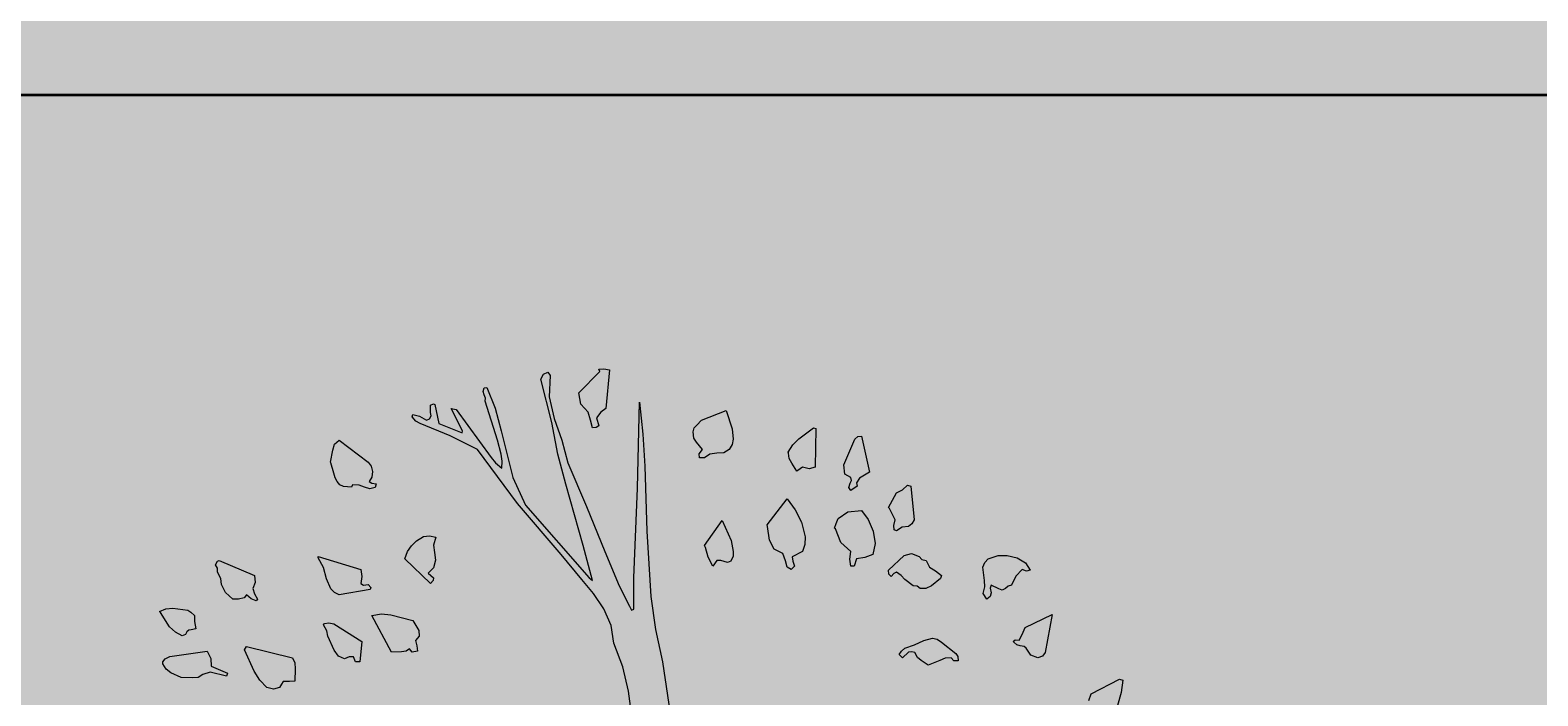
# Model space of a CAD drawing. Units: inches. Extents: x 84 to 1044, y -280 to 906.
# Tile 93 of 105: x 749 to 779, y 499 to 512. Entities that reach past the tile are written whole.
import ezdxf

# ---------------------------------------------------------------- set-up
doc = ezdxf.new("R2010")
doc.units = ezdxf.units.IN
for name, color, linetype, lineweight in [('A-ANNO-DIMS', 2, 'Continuous', 18), ('L-PLNT', 114, 'Continuous', 15), ('WALL', 250, 'Continuous', 35)]:
    doc.layers.add(name, color=color, linetype=linetype, lineweight=lineweight)
doc.layers.add('A-WALL-PATT', color=251, linetype='Continuous', lineweight=9, true_color=0x636466)
doc.layers.add('L-PLNT-PATT', color=9, linetype='Continuous', lineweight=9, true_color=0xafd9aa)
doc.styles.get("Standard").update_dxf_attribs({"font": 'arial.ttf'})
doc.dimstyles.get("Standard").update_dxf_attribs({"dimtxt": 0.18, "dimasz": 0.18, "dimexe": 0.18, "dimexo": 0.0625, "dimgap": 0.09, "dimtad": 0, "dimtih": 1, "dimtoh": 1, "dimdec": 4, "dimzin": 0, "dimdsep": 46, "dimtxsty": 'Standard', "dimcen": 0.09, "dimadec": 0, "dimazin": 0, "dimtfac": 1, "dimtdec": 4, "dimtofl": 0, "dimtmove": 0, "dimatfit": 3, "dimfxl": 1, "dimtolj": 1, "dimtzin": 0, "dimarcsym": 0})

# ---------------------------------------------------------------- blocks, each defined once
blk = doc.blocks.new('A$C37E508DF')
for p, q in [((0.6329, 1.5111), (0.6367, 1.5175)), ((0.6475, 1.4545), (0.6329, 1.5111)), ((0.6367, 1.5175), (0.6423, 1.5201)), ((0.6423, 1.5201), (0.6453, 1.5158)), ((0.6453, 1.5158), (0.644, 1.4879)), ((0.6826, 1.493), (0.7096, 1.5209)), ((0.7083, 1.5239), (0.7152, 1.5244)), ((0.7096, 1.5209), (0.7083, 1.5239)), ((0.7152, 1.5244), (0.7225, 1.5231)), ((0.7225, 1.5231), (0.7174, 1.4729)), ((0.5583, 1.4948), (0.5596, 1.4995)), ((0.5596, 1.4905), (0.5583, 1.4948)), ((0.5596, 1.4995), (0.563, 1.5003)), ((0.5613, 1.4862), (0.5596, 1.4905)), ((0.563, 1.5003), (0.5737, 1.4733)), ((0.6852, 1.4785), (0.6826, 1.493)), ((0.4897, 1.4772), (0.4935, 1.4789)), ((0.4897, 1.4678), (0.4897, 1.4772)), ((0.4935, 1.4789), (0.4952, 1.478)), ((0.4952, 1.478), (0.5004, 1.4532)), ((0.5313, 1.4437), (0.5167, 1.4729)), ((0.5167, 1.4729), (0.5231, 1.4716)), ((0.5231, 1.4716), (0.5686, 1.409)), ((0.5608, 1.4823), (0.5613, 1.4862)), ((0.5767, 1.4317), (0.5608, 1.4823)), ((0.5737, 1.4733), (0.5814, 1.4437)), ((0.644, 1.4879), (0.6505, 1.46)), ((0.6946, 1.4682), (0.6852, 1.4785)), ((0.7174, 1.4729), (0.7109, 1.4682)), ((0.7589, 1.3691), (0.7615, 1.481)), ((0.7615, 1.481), (0.7658, 1.4395)), ((0.8421, 1.4575), (0.8739, 1.4703)), ((0.8739, 1.4703), (0.882, 1.4463)), ((0.4657, 1.4622), (0.4669, 1.4652)), ((0.4708, 1.4566), (0.4657, 1.4622)), ((0.4669, 1.4652), (0.4755, 1.463)), ((0.4764, 1.4532), (0.4708, 1.4566)), ((0.4755, 1.463), (0.4845, 1.4575)), ((0.5154, 1.4373), (0.4764, 1.4532)), ((0.4845, 1.4575), (0.4884, 1.4596)), ((0.4884, 1.4596), (0.4905, 1.4635)), ((0.4905, 1.4635), (0.4897, 1.4678)), ((0.5004, 1.4532), (0.5308, 1.4412)), ((0.6552, 1.4137), (0.6475, 1.4545)), ((0.6505, 1.46), (0.6603, 1.4317)), ((0.6976, 1.4579), (0.6946, 1.4682)), ((0.7002, 1.4476), (0.6976, 1.4579)), ((0.7083, 1.4502), (0.7049, 1.448)), ((0.7109, 1.4682), (0.7053, 1.4609)), ((0.7053, 1.4609), (0.7083, 1.4502)), ((0.8323, 1.4476), (0.8357, 1.451)), ((0.8357, 1.451), (0.8421, 1.4575)), ((0.3649, 1.4266), (0.3709, 1.4317)), ((0.3709, 1.4317), (0.4086, 1.403)), ((0.551, 1.4197), (0.5154, 1.4373)), ((0.5308, 1.4412), (0.5313, 1.4437)), ((0.5814, 1.4133), (0.5767, 1.4317)), ((0.5814, 1.4437), (0.5969, 1.3833)), ((0.6603, 1.4317), (0.668, 1.4021)), ((0.7049, 1.448), (0.7002, 1.4476)), ((0.7658, 1.4395), (0.7684, 1.3979)), ((0.831, 1.4424), (0.8323, 1.4476)), ((0.8318, 1.4343), (0.831, 1.4424)), ((0.8353, 1.4292), (0.8318, 1.4343)), ((0.8829, 1.433), (0.8816, 1.4262)), ((0.882, 1.4463), (0.8829, 1.433)), ((0.9605, 1.4257), (0.9686, 1.4334)), ((0.9686, 1.4334), (0.9875, 1.4476)), ((0.9875, 1.4476), (0.9905, 1.4467)), ((0.9905, 1.4467), (0.9896, 1.3966)), ((1.0269, 1.3996), (1.0411, 1.433)), ((1.0411, 1.433), (1.045, 1.4365)), ((1.045, 1.4365), (1.0497, 1.4369)), ((1.0497, 1.4369), (1.0604, 1.3901)), ((0.3598, 1.403), (0.3628, 1.4189)), ((0.3628, 1.4189), (0.3649, 1.4266)), ((0.6029, 1.3494), (0.551, 1.4197)), ((0.5827, 1.4043), (0.5814, 1.4133)), ((0.6655, 1.3743), (0.6552, 1.4137)), ((0.8434, 1.4197), (0.8353, 1.4292)), ((0.8391, 1.4141), (0.8434, 1.4197)), ((0.8395, 1.4086), (0.8391, 1.4141)), ((0.8528, 1.4137), (0.846, 1.4086)), ((0.8619, 1.4146), (0.8528, 1.4137)), ((0.8709, 1.4154), (0.8619, 1.4146)), ((0.8781, 1.4197), (0.8709, 1.4154)), ((0.8816, 1.4262), (0.8781, 1.4197)), ((0.9545, 1.4159), (0.9605, 1.4257)), ((0.9549, 1.4146), (0.9545, 1.4159)), ((0.9558, 1.4077), (0.9549, 1.4146)), ((0.3602, 1.4021), (0.3598, 1.403)), ((0.364, 1.3888), (0.3602, 1.4021)), ((0.4086, 1.403), (0.4125, 1.3979)), ((0.4125, 1.3979), (0.4142, 1.391)), ((0.5686, 1.409), (0.5741, 1.4021)), ((0.5741, 1.4021), (0.5823, 1.3953)), ((0.5823, 1.3953), (0.5827, 1.4043)), ((0.668, 1.4021), (0.6925, 1.3455)), ((0.7684, 1.3979), (0.771, 1.3134)), ((0.846, 1.4086), (0.8395, 1.4086)), ((0.9592, 1.4017), (0.9558, 1.4077)), ((0.966, 1.3914), (0.9592, 1.4017)), ((0.9703, 1.3944), (0.966, 1.3914)), ((0.9733, 1.3966), (0.9703, 1.3944)), ((0.9819, 1.3944), (0.9733, 1.3966)), ((0.9896, 1.3966), (0.9819, 1.3944)), ((1.0282, 1.3876), (1.0269, 1.3996)), ((0.3657, 1.3828), (0.364, 1.3888)), ((0.3683, 1.3781), (0.3657, 1.3828)), ((0.3718, 1.3738), (0.3683, 1.3781)), ((0.3765, 1.3713), (0.3718, 1.3738)), ((0.3885, 1.3738), (0.3872, 1.3708)), ((0.3971, 1.3734), (0.3885, 1.3738)), ((0.4039, 1.3704), (0.3971, 1.3734)), ((0.4134, 1.3837), (0.4099, 1.3781)), ((0.4099, 1.3781), (0.4134, 1.376)), ((0.4142, 1.391), (0.4134, 1.3837)), ((0.4134, 1.376), (0.4189, 1.3751)), ((0.4189, 1.3751), (0.4176, 1.37)), ((0.5969, 1.3833), (0.6132, 1.3472)), ((0.6882, 1.2949), (0.6655, 1.3743)), ((1.0359, 1.3833), (1.0282, 1.3876)), ((1.0334, 1.37), (1.0351, 1.376)), ((1.0351, 1.376), (1.0368, 1.3794)), ((1.0368, 1.3794), (1.0359, 1.3833)), ((1.0471, 1.3824), (1.0432, 1.3764)), ((1.0432, 1.3764), (1.0441, 1.3717)), ((1.0604, 1.3901), (1.0471, 1.3824)), ((1.1033, 1.367), (1.1097, 1.373)), ((1.1097, 1.373), (1.114, 1.3717)), ((0.3872, 1.3708), (0.3765, 1.3713)), ((0.4108, 1.3683), (0.4039, 1.3704)), ((0.4176, 1.37), (0.4108, 1.3683)), ((0.7538, 1.2529), (0.7589, 1.3691)), ((0.9274, 1.3215), (0.9532, 1.3554)), ((0.9532, 1.3554), (0.9635, 1.3413)), ((1.0359, 1.3661), (1.0334, 1.37)), ((1.0441, 1.3717), (1.0359, 1.3661)), ((1.0848, 1.3443), (1.0955, 1.3631)), ((1.0955, 1.3631), (1.1033, 1.367)), ((1.114, 1.3717), (1.1183, 1.328)), ((0.6595, 1.2829), (0.6029, 1.3494)), ((0.6132, 1.3472), (0.6959, 1.2529)), ((0.6925, 1.3455), (0.7161, 1.2868)), ((0.9635, 1.3413), (0.9721, 1.325)), ((1.0197, 1.3297), (1.0321, 1.3387)), ((1.0321, 1.3387), (1.0497, 1.3404)), ((1.0497, 1.3404), (1.0587, 1.3284)), ((1.0861, 1.343), (1.0848, 1.3443)), ((1.0938, 1.328), (1.0861, 1.343)), ((0.771, 1.3134), (0.7761, 1.2285)), ((0.846, 1.2949), (0.8687, 1.3271)), ((0.8687, 1.3271), (0.8803, 1.3014)), ((0.9279, 1.3194), (0.9274, 1.3215)), ((0.9305, 1.3018), (0.9279, 1.3194)), ((0.9721, 1.325), (0.9768, 1.3061)), ((1.0149, 1.3172), (1.0171, 1.3232)), ((1.0162, 1.3164), (1.0149, 1.3172)), ((1.0231, 1.2988), (1.0162, 1.3164)), ((1.0171, 1.3232), (1.0197, 1.3297)), ((1.0587, 1.3284), (1.0651, 1.3134)), ((1.0651, 1.3134), (1.0677, 1.2975)), ((1.0917, 1.3207), (1.0938, 1.328)), ((1.0925, 1.3151), (1.0917, 1.3207)), ((1.0955, 1.3138), (1.0925, 1.3151)), ((1.1028, 1.3185), (1.0955, 1.3138)), ((1.111, 1.3194), (1.1028, 1.3185)), ((1.1153, 1.3228), (1.111, 1.3194)), ((1.1183, 1.328), (1.1153, 1.3228)), ((0.4597, 1.2868), (0.4648, 1.2945)), ((0.4648, 1.2945), (0.4717, 1.3009)), ((0.4717, 1.3009), (0.4807, 1.3065)), ((0.4807, 1.3065), (0.4884, 1.3074)), ((0.4884, 1.3074), (0.4965, 1.3057)), ((0.4965, 1.3057), (0.4935, 1.2954)), ((0.4935, 1.2954), (0.4948, 1.2855)), ((0.7002, 1.2495), (0.6882, 1.2949)), ((0.8473, 1.2924), (0.846, 1.2949)), ((0.8803, 1.3014), (0.8833, 1.2872)), ((0.9365, 1.2902), (0.9305, 1.3018)), ((0.9763, 1.2962), (0.9733, 1.2868)), ((0.9768, 1.3061), (0.9763, 1.2962)), ((1.0359, 1.2868), (1.0231, 1.2988)), ((1.0677, 1.2975), (1.0647, 1.2829)), ((0.2101, 1.2696), (0.2127, 1.2744)), ((0.2127, 1.2744), (0.2152, 1.2752)), ((0.2152, 1.2752), (0.2611, 1.2559)), ((0.3439, 1.2804), (0.3992, 1.2636)), ((0.3439, 1.2787), (0.3439, 1.2804)), ((0.3507, 1.2662), (0.3439, 1.2787)), ((0.4562, 1.2774), (0.4597, 1.2868)), ((0.4897, 1.2452), (0.4562, 1.2774)), ((0.4961, 1.2756), (0.4935, 1.2658)), ((0.4948, 1.2855), (0.4961, 1.2756)), ((0.6865, 1.2508), (0.6595, 1.2829)), ((0.7161, 1.2868), (0.7349, 1.2422)), ((0.8507, 1.2795), (0.8473, 1.2924)), ((0.8567, 1.2679), (0.8507, 1.2795)), ((0.8619, 1.2752), (0.8567, 1.2679)), ((0.867, 1.2752), (0.8619, 1.2752)), ((0.8713, 1.2739), (0.867, 1.2752)), ((0.8756, 1.2726), (0.8713, 1.2739)), ((0.8799, 1.2744), (0.8756, 1.2726)), ((0.8829, 1.2808), (0.8799, 1.2744)), ((0.8833, 1.2872), (0.8829, 1.2808)), ((0.9476, 1.2842), (0.9365, 1.2902)), ((0.951, 1.2748), (0.9476, 1.2842)), ((0.9532, 1.2666), (0.951, 1.2748)), ((0.9733, 1.2868), (0.9596, 1.2799)), ((0.9596, 1.2799), (0.9605, 1.2744)), ((0.9605, 1.2744), (0.9626, 1.2679)), ((1.0347, 1.2769), (1.0359, 1.2868)), ((1.0359, 1.2679), (1.0347, 1.2769)), ((1.0432, 1.2774), (1.0402, 1.2679)), ((1.0544, 1.2791), (1.0432, 1.2774)), ((1.0647, 1.2829), (1.0544, 1.2791)), ((1.0848, 1.2628), (1.1054, 1.2817)), ((1.1054, 1.2817), (1.1148, 1.2842)), ((1.1148, 1.2842), (1.1247, 1.2804)), ((1.1247, 1.2804), (1.1281, 1.2765)), ((1.1281, 1.2765), (1.1341, 1.2752)), ((1.1341, 1.2752), (1.1384, 1.2666)), ((1.21, 1.2726), (1.2147, 1.2774)), ((1.2147, 1.2774), (1.2276, 1.2817)), ((1.2276, 1.2817), (1.2392, 1.2817)), ((1.2392, 1.2817), (1.2521, 1.2787)), ((1.2521, 1.2787), (1.2632, 1.2722)), ((0.2127, 1.2654), (0.2101, 1.2696)), ((0.2127, 1.2602), (0.2127, 1.2654)), ((0.2174, 1.2521), (0.2127, 1.2602)), ((0.2611, 1.2559), (0.262, 1.2465)), ((0.3546, 1.2516), (0.3507, 1.2662)), ((0.3992, 1.2636), (0.4005, 1.2546)), ((0.4005, 1.2546), (0.3992, 1.2452)), ((0.4935, 1.2658), (0.4867, 1.2589)), ((0.4867, 1.2589), (0.4935, 1.2529)), ((0.9583, 1.2636), (0.9532, 1.2666)), ((0.9626, 1.2679), (0.9583, 1.2636)), ((1.0402, 1.2679), (1.0359, 1.2679)), ((1.0852, 1.2576), (1.0848, 1.2628)), ((1.0883, 1.2546), (1.0852, 1.2576)), ((1.0921, 1.2585), (1.0883, 1.2546)), ((1.0955, 1.2602), (1.0921, 1.2585)), ((1.1015, 1.2559), (1.0955, 1.2602)), ((1.1063, 1.2508), (1.1015, 1.2559)), ((1.1384, 1.2666), (1.1461, 1.2619)), ((1.1461, 1.2619), (1.1539, 1.2559)), ((1.1539, 1.2559), (1.1526, 1.2521)), ((1.2075, 1.2666), (1.21, 1.2726)), ((1.2096, 1.2491), (1.2075, 1.2666)), ((1.2503, 1.2551), (1.2448, 1.2431)), ((1.2585, 1.2636), (1.2503, 1.2551)), ((1.2645, 1.2615), (1.2585, 1.2636)), ((1.2632, 1.2722), (1.2692, 1.2628)), ((1.2692, 1.2628), (1.2645, 1.2615)), ((0.2182, 1.2443), (0.2174, 1.2521)), ((0.2234, 1.2336), (0.2182, 1.2443)), ((0.262, 1.2465), (0.2586, 1.2388)), ((0.2586, 1.2388), (0.2611, 1.2319)), ((0.3602, 1.2383), (0.3546, 1.2516)), ((0.3649, 1.2336), (0.3602, 1.2383)), ((0.4112, 1.2375), (0.3709, 1.2306)), ((0.3992, 1.2452), (0.4026, 1.2431)), ((0.4026, 1.2431), (0.4086, 1.2443)), ((0.4086, 1.2443), (0.4121, 1.2401)), ((0.4121, 1.2401), (0.4112, 1.2375)), ((0.4931, 1.2491), (0.4897, 1.2452)), ((0.4935, 1.2529), (0.4931, 1.2491)), ((0.7015, 1.2323), (0.6865, 1.2508)), ((0.6959, 1.2529), (0.7002, 1.2495)), ((0.7349, 1.2422), (0.7482, 1.216)), ((0.7538, 1.2122), (0.7538, 1.2529)), ((1.117, 1.2422), (1.1063, 1.2508)), ((1.1221, 1.2418), (1.117, 1.2422)), ((1.126, 1.2388), (1.1221, 1.2418)), ((1.1337, 1.2388), (1.126, 1.2388)), ((1.141, 1.2422), (1.1337, 1.2388)), ((1.1526, 1.2521), (1.141, 1.2422)), ((1.2079, 1.2323), (1.21, 1.2409)), ((1.21, 1.2409), (1.2096, 1.2491)), ((1.2186, 1.2431), (1.2173, 1.2392)), ((1.2173, 1.2392), (1.2186, 1.2332)), ((1.2285, 1.2383), (1.2186, 1.2431)), ((1.2328, 1.2366), (1.2285, 1.2383)), ((1.2371, 1.2388), (1.2328, 1.2366)), ((1.2405, 1.2418), (1.2371, 1.2388)), ((1.2448, 1.2431), (1.2405, 1.2418)), ((0.2328, 1.2251), (0.2234, 1.2336)), ((0.2401, 1.2251), (0.2328, 1.2251)), ((0.2474, 1.2268), (0.2401, 1.2251)), ((0.2504, 1.2306), (0.2474, 1.2268)), ((0.2568, 1.2255), (0.2504, 1.2306)), ((0.2633, 1.2229), (0.2568, 1.2255)), ((0.2611, 1.2319), (0.265, 1.2251)), ((0.265, 1.2251), (0.2633, 1.2229)), ((0.3709, 1.2306), (0.3649, 1.2336)), ((0.7148, 1.2126), (0.7015, 1.2323)), ((0.7482, 1.216), (0.7508, 1.2109)), ((0.7761, 1.2285), (0.7821, 1.1856)), ((1.2126, 1.2251), (1.2079, 1.2323)), ((1.2169, 1.2285), (1.2126, 1.2251)), ((1.2186, 1.2332), (1.2169, 1.2285)), ((0.1376, 1.2092), (0.1458, 1.2126)), ((0.1389, 1.2079), (0.1376, 1.2092)), ((0.1505, 1.189), (0.1389, 1.2079)), ((0.1458, 1.2126), (0.1548, 1.2135)), ((0.1548, 1.2135), (0.1741, 1.2109)), ((0.1741, 1.2109), (0.1784, 1.2083)), ((0.1784, 1.2083), (0.1831, 1.204)), ((0.1831, 1.204), (0.1831, 1.1959)), ((0.1831, 1.1959), (0.1848, 1.1865)), ((0.4134, 1.204), (0.4258, 1.2058)), ((0.4391, 1.156), (0.4134, 1.204)), ((0.4258, 1.2058), (0.4382, 1.2045)), ((0.4382, 1.2045), (0.4669, 1.1972)), ((0.4669, 1.1972), (0.4747, 1.1843)), ((0.7246, 1.1908), (0.7148, 1.2126)), ((0.7508, 1.2109), (0.7538, 1.2122)), ((1.2628, 1.1882), (1.2975, 1.2053)), ((1.2975, 1.2053), (1.2885, 1.1556)), ((0.1582, 1.1822), (0.1505, 1.189)), ((0.1668, 1.1775), (0.1582, 1.1822)), ((0.1711, 1.1792), (0.1668, 1.1775)), ((0.1728, 1.1826), (0.1711, 1.1792)), ((0.1758, 1.1847), (0.1728, 1.1826)), ((0.1788, 1.1852), (0.1758, 1.1847)), ((0.1848, 1.1865), (0.1788, 1.1852)), ((0.3507, 1.1916), (0.352, 1.1933)), ((0.355, 1.1839), (0.3507, 1.1916)), ((0.352, 1.1933), (0.3576, 1.1942)), ((0.3563, 1.177), (0.355, 1.1839)), ((0.3645, 1.1586), (0.3563, 1.177)), ((0.3576, 1.1942), (0.364, 1.1929)), ((0.364, 1.1929), (0.4005, 1.1702)), ((0.4751, 1.177), (0.47, 1.1714)), ((0.4747, 1.1843), (0.4751, 1.177)), ((0.7281, 1.168), (0.7246, 1.1908)), ((0.7821, 1.1856), (0.7911, 1.1436)), ((1.2546, 1.1719), (1.2589, 1.1792)), ((1.2589, 1.1792), (1.2628, 1.1882)), ((0.1509, 1.1504), (0.1994, 1.1573)), ((0.1994, 1.1573), (0.2041, 1.1479)), ((0.2478, 1.1594), (0.2504, 1.1637)), ((0.2607, 1.1316), (0.2478, 1.1594)), ((0.2504, 1.1637), (0.3104, 1.1487)), ((0.37, 1.1509), (0.3645, 1.1586)), ((0.4005, 1.1702), (0.3979, 1.1436)), ((0.4519, 1.1564), (0.4391, 1.156)), ((0.458, 1.1573), (0.4519, 1.1564)), ((0.4622, 1.1607), (0.458, 1.1573)), ((0.4657, 1.156), (0.4622, 1.1607)), ((0.473, 1.1573), (0.4657, 1.156)), ((0.47, 1.1714), (0.4721, 1.1646)), ((0.4721, 1.1646), (0.473, 1.1573)), ((0.7396, 1.1371), (0.7281, 1.168)), ((1.099, 1.153), (1.102, 1.1573)), ((1.102, 1.1573), (1.1063, 1.1612)), ((1.1063, 1.1612), (1.1187, 1.1655)), ((1.1153, 1.1564), (1.111, 1.156)), ((1.1191, 1.1556), (1.1153, 1.1564)), ((1.1187, 1.1655), (1.1307, 1.1714)), ((1.1307, 1.1714), (1.1423, 1.1744)), ((1.1423, 1.1744), (1.1483, 1.1732)), ((1.1483, 1.1732), (1.1539, 1.1693)), ((1.1539, 1.1693), (1.1727, 1.1543)), ((1.2469, 1.1702), (1.2495, 1.1723)), ((1.2478, 1.1693), (1.2469, 1.1702)), ((1.2516, 1.1659), (1.2478, 1.1693)), ((1.2495, 1.1723), (1.2546, 1.1719)), ((1.2563, 1.1646), (1.2516, 1.1659)), ((1.2611, 1.1637), (1.2563, 1.1646)), ((1.2641, 1.1612), (1.2611, 1.1637)), ((1.2701, 1.1522), (1.2641, 1.1612)), ((0.1419, 1.1436), (0.1449, 1.1474)), ((0.1419, 1.141), (0.1419, 1.1436)), ((0.1462, 1.1342), (0.1419, 1.141)), ((0.1449, 1.1474), (0.1509, 1.1504)), ((0.2041, 1.1479), (0.2045, 1.138)), ((0.2045, 1.138), (0.226, 1.129)), ((0.3104, 1.1487), (0.3134, 1.1423)), ((0.3134, 1.1423), (0.3139, 1.1346)), ((0.3778, 1.1474), (0.37, 1.1509)), ((0.3842, 1.15), (0.3778, 1.1474)), ((0.3898, 1.15), (0.3842, 1.15)), ((0.3923, 1.1436), (0.3898, 1.15)), ((0.3979, 1.1436), (0.3923, 1.1436)), ((0.7469, 1.1054), (0.7396, 1.1371)), ((0.7911, 1.1436), (0.8027, 1.0677)), ((1.1033, 1.1487), (1.099, 1.153)), ((1.111, 1.156), (1.1033, 1.1487)), ((1.1226, 1.1492), (1.1191, 1.1556)), ((1.1273, 1.1453), (1.1226, 1.1492)), ((1.1367, 1.1393), (1.1273, 1.1453)), ((1.1517, 1.1453), (1.1367, 1.1393)), ((1.1586, 1.1483), (1.1517, 1.1453)), ((1.1663, 1.1487), (1.1586, 1.1483)), ((1.1697, 1.1449), (1.1663, 1.1487)), ((1.1757, 1.1449), (1.1697, 1.1449)), ((1.1727, 1.1543), (1.1749, 1.1504)), ((1.1749, 1.1504), (1.1757, 1.1449)), ((1.2791, 1.1487), (1.2701, 1.1522)), ((1.2851, 1.1509), (1.2791, 1.1487)), ((1.2885, 1.1556), (1.2851, 1.1509)), ((0.1522, 1.1294), (0.1462, 1.1342)), ((0.1655, 1.1234), (0.1522, 1.1294)), ((0.181, 1.1226), (0.1655, 1.1234)), ((0.1878, 1.1234), (0.181, 1.1226)), ((0.1938, 1.1273), (0.1878, 1.1234)), ((0.2032, 1.1303), (0.1938, 1.1273)), ((0.2247, 1.1251), (0.2032, 1.1303)), ((0.226, 1.129), (0.2247, 1.1251)), ((0.268, 1.1196), (0.2607, 1.1316)), ((0.277, 1.1101), (0.268, 1.1196)), ((0.2984, 1.1179), (0.2959, 1.1144)), ((0.3066, 1.1179), (0.2984, 1.1179)), ((0.3134, 1.1183), (0.3066, 1.1179)), ((0.3139, 1.1346), (0.3134, 1.1183)), ((1.3485, 1.102), (1.385, 1.1209)), ((1.385, 1.1209), (1.3897, 1.1196)), ((1.3897, 1.1196), (1.3875, 1.1037)), ((0.2856, 1.108), (0.277, 1.1101)), ((0.2933, 1.1101), (0.2856, 1.108)), ((0.2959, 1.1144), (0.2933, 1.1101)), ((0.7512, 1.0728), (0.7469, 1.1054)), ((1.3455, 1.0934), (1.3485, 1.102)), ((1.3875, 1.1037), (1.3828, 1.087))]:
    blk.add_line(p, q)
blk = doc.blocks.new('*D62')
at = {"layer": 'A-ANNO-DIMS', "color": 0, "lineweight": -2, "transparency": 16777216}
for p, q in [((203.179, 709.183), (203.179, 905.9)), ((896.074, 400.183), (896.074, 905.9)), ((203.359, 905.72), (549.232, 905.72)), ((895.894, 905.72), (550.021, 905.72))]:
    blk.add_line(p, q, dxfattribs=at)
at = {"layer": 'A-ANNO-DIMS', "color": 0, "transparency": 16777216}
for points in [[(203.359, 905.75), (203.359, 905.69), (203.179, 905.72)], [(895.894, 905.75), (895.894, 905.69), (896.074, 905.72)]]:
    blk.add_solid(points, dxfattribs=at)
at = {"layer": 'Defpoints', "color": 0, "transparency": 16777216}
for p in [(896.074, 905.72), (203.179, 709.12), (896.074, 400.12)]:
    blk.add_point(p, dxfattribs=at)
at = {"layer": 'A-ANNO-DIMS', "color": 0, "transparency": 16777216, "insert": (549.627, 905.72), "char_height": 0.18, "attachment_point": 5}
blk.add_mtext('\\A1;692.9', dxfattribs=at)

msp = doc.modelspace()

# ---------------------------------------------------------------- hatches: boundary and pattern name
at = {"layer": 'A-WALL-PATT', "transparency": 33554597}
h = msp.add_hatch(color=256, dxfattribs=at)
h.dxf.hatch_style = 1
h.paths.add_polyline_path([(671.074, 100.12), (647.074, 100.12), (647.074, 160.12), (641.074, 160.12), (620.824, 160.12), (620.824, 151.12), (638.074, 151.12), (638.074, 91.12), (671.074, 91.12)])
h.paths.add_polyline_path([(791.074, 100.12), (743.074, 100.12), (743.074, 91.12), (791.074, 91.12)])
h.paths.add_polyline_path([(896.074, 346.12), (887.074, 346.12), (887.074, 334.12), (870.955, 334.12), (833.074, 334.12), (804.574, 334.12), (804.574, 328.12), (887.074, 328.12), (887.074, 100.12), (863.074, 100.12), (863.074, 91.12), (896.074, 91.12)])
h.paths.add_polyline_path([(507.574, 154.729), (507.574, 160.12), (464.074, 160.12), (464.074, 247.12), (641.074, 247.12), (641.074, 208.12), (647.074, 208.12), (647.074, 328.12), (659.074, 328.12), (659.074, 334.12), (617.074, 334.12), (617.074, 328.12), (641.074, 328.12), (641.074, 256.12), (545.074, 256.12), (545.074, 328.12), (569.074, 328.12), (569.074, 334.12), (518.074, 334.12), (518.074, 325.12), (536.074, 325.12), (536.074, 256.12), (464.074, 256.12), (464.074, 325.12), (482.074, 325.12), (482.074, 334.12), (455.074, 334.12), (455.074, 160.12), (413.127, 160.12), (413.127, 151.12), (455.074, 151.12), (455.074, 91.12), (464.074, 91.12), (464.074, 151.12), (507.574, 151.12)])
h.paths.add_polyline_path([(572.824, 160.12), (555.574, 160.12), (555.574, 151.12), (572.824, 151.12)], flags=17)
h.paths.add_polyline_path([(341.127, 160.12), (299.179, 160.12), (299.179, 211.12), (294.179, 211.12), (290.179, 211.12), (290.179, 151.12), (341.127, 151.12)])
h.paths.add_polyline_path([(299.179, 256.12), (212.179, 256.12), (212.179, 274.12), (203.179, 274.12), (203.179, 247.12), (299.179, 247.12)])
h.paths.add_polyline_path([(212.179, 514.12), (398.074, 514.12), (398.074, 519.12), (398.074, 520.12), (212.179, 520.12), (212.179, 574.12), (203.179, 574.12), (203.179, 310.12), (212.179, 310.12), (212.179, 328.12), (290.179, 328.12), (290.179, 292.12), (299.179, 292.12), (299.179, 328.12), (332.179, 328.12), (332.179, 334.12), (212.179, 334.12)])
h.paths.add_polyline_path([(287.127, 709.12), (203.179, 709.12), (203.179, 646.12), (212.179, 646.12), (212.179, 700.12), (287.127, 700.12)])
h.paths.add_polyline_path([(470.074, 709.12), (359.127, 709.12), (359.127, 700.12), (434.074, 700.12), (434.074, 574.12), (440.074, 574.12), (440.074, 622.12), (464.074, 622.12), (464.074, 628.12), (440.074, 628.12), (440.074, 700.12), (470.074, 700.12)])
h.paths.add_polyline_path([(572.074, 709.12), (506.074, 709.12), (506.074, 700.12), (536.074, 700.12), (536.074, 628.12), (494.074, 628.12), (494.074, 622.12), (536.074, 622.12), (536.074, 520.12), (440.074, 520.12), (440.074, 544.12), (434.074, 544.12), (434.074, 514.12), (644.074, 514.12), (644.074, 519.12), (644.074, 544.12), (638.074, 544.12), (638.074, 520.12), (542.074, 520.12), (542.074, 622.12), (584.074, 622.12), (584.074, 628.12), (542.074, 628.12), (542.074, 700.12), (572.074, 700.12)])
h.paths.add_polyline_path([(698.074, 709.12), (608.074, 709.12), (608.074, 700.12), (638.074, 700.12), (638.074, 628.12), (614.074, 628.12), (614.074, 622.12), (638.074, 622.12), (638.074, 574.12), (644.074, 574.12), (644.074, 700.12), (698.074, 700.12)])
h.paths.add_polyline_path([(833.074, 709.12), (770.074, 709.12), (770.074, 700.12), (824.074, 700.12), (824.074, 646.12), (833.074, 646.12)])
h.paths.add_polyline_path([(833.074, 574.12), (824.074, 574.12), (824.074, 520.12), (791.244, 520.12), (712.904, 520.12), (680.074, 520.12), (680.074, 514.12), (695.074, 514.12), (695.074, 491.62), (704.074, 491.62), (704.074, 511.12), (833.074, 511.12)])
h.paths.add_polyline_path([(704.074, 419.62), (695.074, 419.62), (695.074, 370.12), (704.074, 370.12)])
h.paths.add_polyline_path([(896.074, 400.12), (833.074, 400.12), (833.074, 364.12), (839.074, 364.12), (839.074, 394.12), (887.074, 394.12), (887.074, 382.12), (896.074, 382.12)])
h.paths.add_polyline_path([(732.574, 334.12), (695.074, 334.12), (695.074, 328.12), (732.574, 328.12)])
at = {"layer": 'L-PLNT-PATT', "transparency": 33554597}
h = msp.add_hatch(color=256, dxfattribs=at)
h.dxf.hatch_style = 1
h.paths.add_polyline_path([(896.074, 511.12), (704.074, 511.12), (704.074, 491.62), (704.074, 419.62), (704.074, 400.12), (833.074, 400.12), (896.074, 400.12)])

# ---------------------------------------------------------------- linework, layer by layer
at = {"layer": 'WALL'}
msp.add_line((896.074, 511.12), (704.074, 511.12), dxfattribs=at)

# ---------------------------------------------------------------- block references
at = {"layer": 'L-PLNT', "xscale": 15.19586232982809, "yscale": 15.19586232982809, "zscale": 15.19586232982809}
msp.add_blockref('A$C37E508DF', (749.806, 482.553), dxfattribs=at)

# ---------------------------------------------------------------- dimensions: what is measured, and where the dimension line sits
at = {"layer": 'A-ANNO-DIMS'}
dim = msp.add_linear_dim(base=(896.074, 905.72), p1=(203.179, 709.12), p2=(896.074, 400.12), dimstyle='Standard', override={"dimdec": 1, "dimlfac": 1, "dimrnd": 0, "dimzin": 0, "dimdsep": 46, "dimlunit": 2}, dxfattribs=at)
dim.commit()
dim.dimension.update_dxf_attribs({"geometry": '*D62', "text_midpoint": (549.627, 905.72)})

doc.saveas('drawing.dxf')
